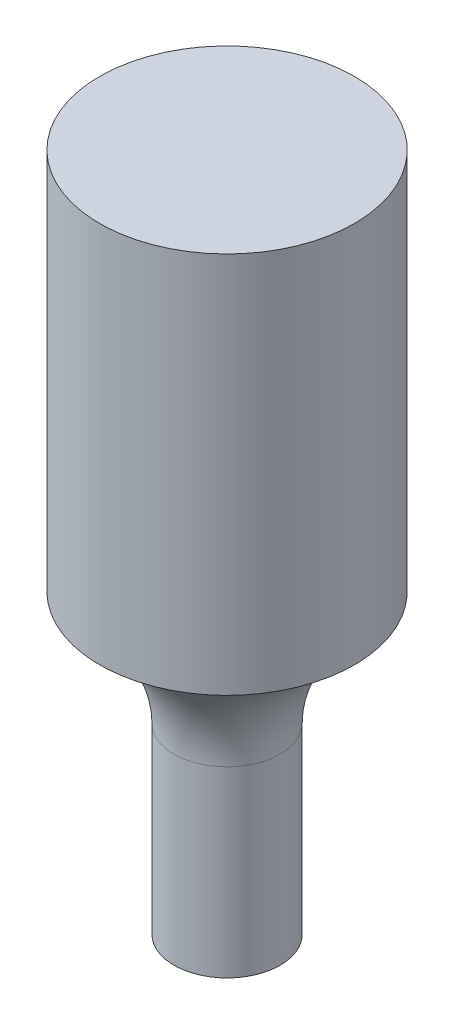
from build123d import *


with BuildPart() as part:
    # Punch Profile Sketch → Punch Body Revolve (revolve)
    with BuildSketch(Plane.XY, mode=Mode.PRIVATE) as punch_body_revolve_sk:
        with BuildLine():
            Line((0, 0), (-2.5, 0))
            Line((-2.5, 0), (-2.5, 8.610194809))
            ThreePointArc((-2.5, 8.610194809), (-3.451767993, 11.823448611), (-6, 14))
            Line((-6, 14), (-6, 32))
            Line((-6, 32), (0, 32))
            Line((0, 32), (0, 0))
        make_face()
    revolve(punch_body_revolve_sk.sketch.rotate(Axis((0, 0, 0), (0, 1, 0)), 270), axis=Axis((0, 0, 0), (0, 1, 0)))


solid = part.part
